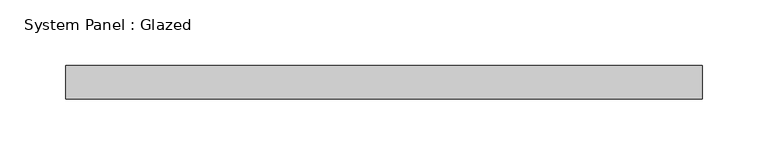
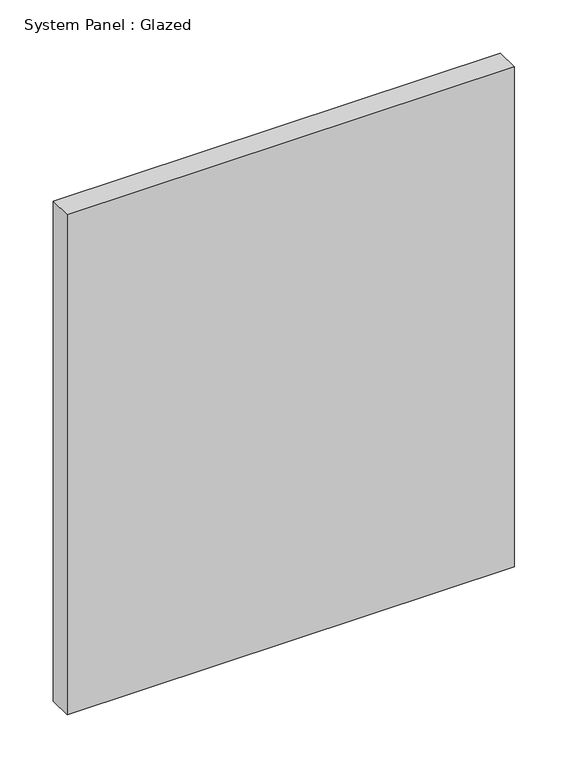
"""IFC4 building model written with IfcOpenShell, lengths in millimetres: plate geometry, System Panel : Glazed."""

from ifc_helpers import new_model, si_unit, origin, origin_with_axes, place, context, project, spatial, polyline, outline, extrude, source, transform, mapped, element, save


def system_panel_glazed_f3433a31(model_context):
    return source(origin(), model_context, "Body", "SweptSolid", [
        extrude(outline(polyline([(241.3, 19.05), (-241.3, 19.05), (-241.3, 44.45), (241.3, 44.45), (241.3, 19.05)])), origin_with_axes(), (0.0, 0.0, 1.0), 570.2142589),
    ])


if __name__ == "__main__":
    model = new_model("IFC4")
    model_context = context("Model", 3, world=origin())
    ifc_project = project(units=[si_unit("LENGTHUNIT", "METRE", prefix="MILLI")], contexts=[model_context])
    site = spatial("IfcSite", under=ifc_project)
    building = spatial("IfcBuilding", under=site)
    placement = place(None, origin())
    system_panel_glazed_shape = system_panel_glazed_f3433a31(model_context)
    element("IfcPlate", 1, ObjectType="System Panel : Glazed", at=placement, inside=building, context=model_context, shape_type="MappedRepresentation", body=[
        mapped(system_panel_glazed_shape, transform((0.0, 0.0, 0.0), x_axis=(1.0, 0.0, 0.0), y_axis=(0.0, 1.0, 0.0), z_axis=(0.0, 0.0, 1.0))),
    ])
    save(model, "model.ifc")

# Revit data of these elements
# Type "System Panel : Glazed"
#   Construction Type Id = "GSP4R"
#   Analytic Construction = "1/8 in Pilkington single glazing"
#   Visual Light Transmittance = 0.9
#   Solar Heat Gain Coefficient = 0.86
#   Heat Transfer Coefficient (U) = 1.18115 BTU/(h·ft²·°F)
#   Define Thermal Properties by = 1
# Element 1 (IfcPlate, "System Panel : Glazed")
#   Materials on its faces: "Glass"
# Materials
#   "Glass": class "Glass", colour RGB 0 128 192, transparency 0.75, Description = "Soda Lime Glass", Cost = 0
